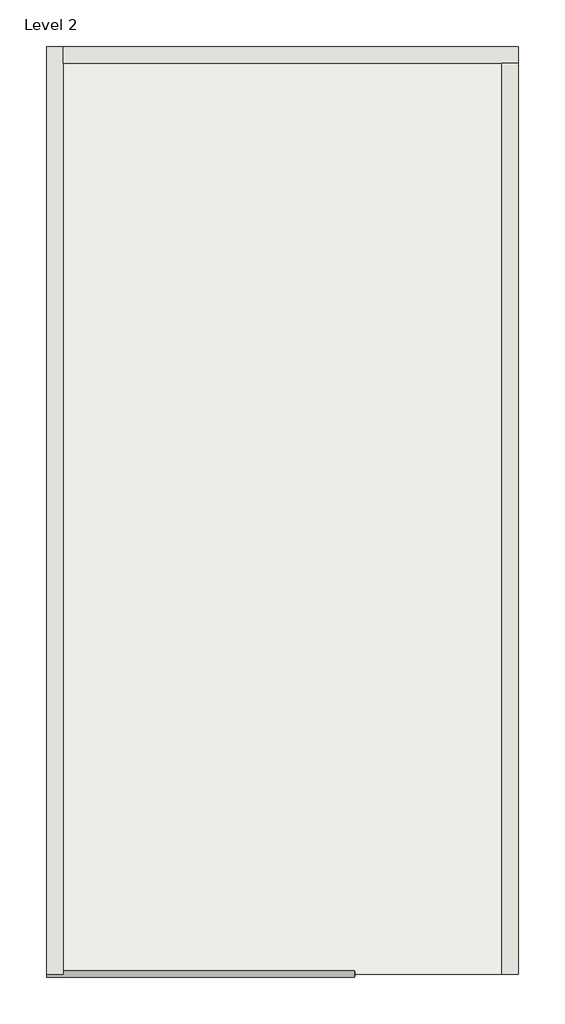
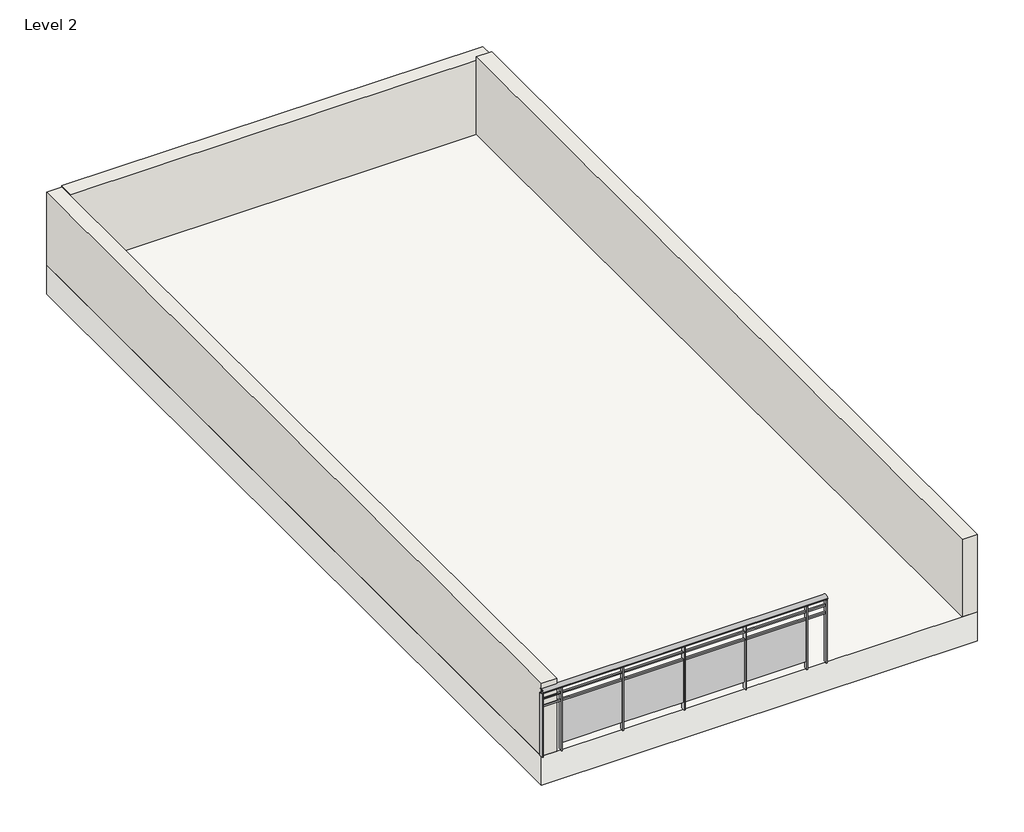
# One storey: 3 walls, 1 railing, 1 slab.
"""IFC4 building model written with IfcOpenShell, lengths in millimetres."""

from ifc_helpers import new_model, si_unit, point, frame, origin, place, context, project, spatial, polyline, ellipse_curve, trimmed, outline, extrude, faceted_brep, element, save
from ifc_brep_helpers import plane_surface, extruded_surface, advanced_brep

model = new_model("IFC4")

# Units and contexts
model_context = context("Model", 3, world=origin())
ifc_project = project(units=[si_unit("LENGTHUNIT", "METRE", prefix="MILLI")], contexts=[model_context])

# Site, building, storey
site = spatial("IfcSite", under=ifc_project)
building = spatial("IfcBuilding", under=site)
storey = spatial("IfcBuildingStorey", under=building, Name="Level 2", Elevation=6096.0)

# Railing
placement = place(None, origin())
element("IfcRailing", 1, ObjectType="Glass Panel - Bottom Fill", at=placement, inside=storey, context=model_context, shape_type="SolidModel", body=[
    advanced_brep(
    [(-9880.3407032, 3900.3863751, 6996.0), (-9880.3407032, 3820.3863751, 6996.0), (-6171.9407032, 3900.3863751, 6996.0), (-6171.9407032, 3820.3863751, 6996.0)],
    [
        (0, 1, ellipse_curve(frame((-9880.3407032, 3860.3863751, 6996.0), z_axis=(-1.0, 0.0, 0.0), x_axis=(0.0, -1.0, 0.0)), 40.0, 30.0)),
        (1, 0, ellipse_curve(frame((-9880.3407032, 3860.3863751, 6996.0), z_axis=(-1.0, 0.0, 0.0), x_axis=(0.0, -1.0, 0.0)), 40.0, 30.0)),
        (2, 3, ellipse_curve(frame((-6171.9407032, 3860.3863751, 6996.0), z_axis=(1.0, 0.0, 0.0), x_axis=(0.0, -1.0, 0.0)), 40.0, 30.0)),
        (3, 2, ellipse_curve(frame((-6171.9407032, 3860.3863751, 6996.0), z_axis=(1.0, 0.0, 0.0), x_axis=(0.0, -1.0, 0.0)), 40.0, 30.0)),
        (0, 2),
        (3, 1),
    ],
    [
        plane_surface(frame((-9880.3407032, 3860.3863751, 6996.0), z_axis=(-1.0, 0.0, 0.0), x_axis=(0.0, 1.0, 0.0))),
        plane_surface(frame((-6171.9407032, 3860.3863751, 6996.0), z_axis=(1.0, 0.0, 0.0), x_axis=(0.0, 1.0, 0.0))),
        extruded_surface(trimmed(ellipse_curve(frame((-6171.9407032, 3860.3863751, 6996.0), z_axis=(-1.0, 0.0, 0.0), x_axis=(0.0, -1.0, 0.0)), 40.0, 30.0), [point((-6171.9407032, 3900.3863751, 6996.0))], [point((-6171.9407032, 3820.3863751, 6996.0))], True, "CARTESIAN"), (-3708.3999999999996, 0.0, 0.0), 3708.3999999999996),
        extruded_surface(trimmed(ellipse_curve(frame((-6171.9407032, 3860.3863751, 6996.0), z_axis=(-1.0, 0.0, 0.0), x_axis=(0.0, -1.0, 0.0)), 40.0, 30.0), [point((-6171.9407032, 3820.3863751, 6996.0))], [point((-6171.9407032, 3900.3863751, 6996.0))], True, "CARTESIAN"), (-3708.3999999999996, 0.0, 0.0), 3708.3999999999996),
    ],
    [
        (0, [[1, 2]]),
        (1, [[3, 4]]),
        (2, [[-1, 5, -4, 6]]),
        (3, [[-2, -6, -3, -5]]),
    ],
),
    extrude(outline(polyline([(-9880.3407032, 3850.9956099), (-9880.3407032, 3870.9956099), (-6171.9407032, 3870.9956099), (-6171.9407032, 3850.9956099), (-9880.3407032, 3850.9956099)])), frame((0.0, 0.0, 6876.0), z_axis=(0.0, 0.0, 1.0), x_axis=(1.0, 0.0, 0.0)), (0.0, 0.0, 1.0), 20.0),
    extrude(outline(polyline([(-9880.3407032, 3850.9956099), (-9880.3407032, 3870.9956099), (-6171.9407032, 3870.9956099), (-6171.9407032, 3850.9956099), (-9880.3407032, 3850.9956099)])), frame((0.0, 0.0, 6776.0), z_axis=(0.0, 0.0, 1.0), x_axis=(1.0, 0.0, 0.0)), (0.0, 0.0, 1.0), 20.0),
    extrude(outline(polyline([(-6432.1407032, 3885.9956099), (-6420.1407032, 3885.9956099), (-6420.1407032, 3835.9956099), (-6432.1407032, 3835.9956099), (-6432.1407032, 3885.9956099)])), frame((0.0, 0.0, 6096.0), z_axis=(0.0, 0.0, 1.0), x_axis=(1.0, 0.0, 0.0)), (0.0, 0.0, 1.0), 869.8465326),
    extrude(outline(polyline([(-7226.1407032, 3859.2707998), (-6426.1407032, 3859.2707998), (-6426.1407032, 3854.2707998), (-7226.1407032, 3854.2707998), (-7226.1407032, 3859.2707998)])), frame((0.0, 0.0, 6196.0), z_axis=(0.0, 0.0, 1.0), x_axis=(1.0, 0.0, 0.0)), (0.0, 0.0, 1.0), 580.0),
    extrude(outline(polyline([(-7232.1407032, 3885.9956099), (-7220.1407032, 3885.9956099), (-7220.1407032, 3835.9956099), (-7232.1407032, 3835.9956099), (-7232.1407032, 3885.9956099)])), frame((0.0, 0.0, 6096.0), z_axis=(0.0, 0.0, 1.0), x_axis=(1.0, 0.0, 0.0)), (0.0, 0.0, 1.0), 869.8465326),
    extrude(outline(polyline([(-8026.1407032, 3859.2707998), (-7226.1407032, 3859.2707998), (-7226.1407032, 3854.2707998), (-8026.1407032, 3854.2707998), (-8026.1407032, 3859.2707998)])), frame((0.0, 0.0, 6196.0), z_axis=(0.0, 0.0, 1.0), x_axis=(1.0, 0.0, 0.0)), (0.0, 0.0, 1.0), 580.0),
    extrude(outline(polyline([(-8032.1407032, 3885.9956099), (-8020.1407032, 3885.9956099), (-8020.1407032, 3835.9956099), (-8032.1407032, 3835.9956099), (-8032.1407032, 3885.9956099)])), frame((0.0, 0.0, 6096.0), z_axis=(0.0, 0.0, 1.0), x_axis=(1.0, 0.0, 0.0)), (0.0, 0.0, 1.0), 869.8465326),
    extrude(outline(polyline([(-8826.1407032, 3859.2707998), (-8026.1407032, 3859.2707998), (-8026.1407032, 3854.2707998), (-8826.1407032, 3854.2707998), (-8826.1407032, 3859.2707998)])), frame((0.0, 0.0, 6196.0), z_axis=(0.0, 0.0, 1.0), x_axis=(1.0, 0.0, 0.0)), (0.0, 0.0, 1.0), 580.0),
    extrude(outline(polyline([(-8832.1407032, 3885.9956099), (-8820.1407032, 3885.9956099), (-8820.1407032, 3835.9956099), (-8832.1407032, 3835.9956099), (-8832.1407032, 3885.9956099)])), frame((0.0, 0.0, 6096.0), z_axis=(0.0, 0.0, 1.0), x_axis=(1.0, 0.0, 0.0)), (0.0, 0.0, 1.0), 869.8465326),
    extrude(outline(polyline([(-9626.1407032, 3859.2707998), (-8826.1407032, 3859.2707998), (-8826.1407032, 3854.2707998), (-9626.1407032, 3854.2707998), (-9626.1407032, 3859.2707998)])), frame((0.0, 0.0, 6196.0), z_axis=(0.0, 0.0, 1.0), x_axis=(1.0, 0.0, 0.0)), (0.0, 0.0, 1.0), 580.0),
    extrude(outline(polyline([(-9632.1407032, 3885.9956099), (-9620.1407032, 3885.9956099), (-9620.1407032, 3835.9956099), (-9632.1407032, 3835.9956099), (-9632.1407032, 3885.9956099)])), frame((0.0, 0.0, 6096.0), z_axis=(0.0, 0.0, 1.0), x_axis=(1.0, 0.0, 0.0)), (0.0, 0.0, 1.0), 869.8465326),
    extrude(outline(polyline([(-6179.9407032, 3885.9956099), (-6167.9407032, 3885.9956099), (-6167.9407032, 3835.9956099), (-6179.9407032, 3835.9956099), (-6179.9407032, 3885.9956099)])), frame((0.0, 0.0, 6096.0), z_axis=(0.0, 0.0, 1.0), x_axis=(1.0, 0.0, 0.0)), (0.0, 0.0, 1.0), 869.8465326),
    extrude(outline(polyline([(-9884.3407032, 3885.9956099), (-9872.3407032, 3885.9956099), (-9872.3407032, 3835.9956099), (-9884.3407032, 3835.9956099), (-9884.3407032, 3885.9956099)])), frame((0.0, 0.0, 6096.0), z_axis=(0.0, 0.0, 1.0), x_axis=(1.0, 0.0, 0.0)), (0.0, 0.0, 1.0), 869.8465326),
])

# Slab
element("IfcSlab", 2, ObjectType="Generic Floor - 400mm", at=placement, inside=storey, context=model_context, shape_type="SweptSolid", body=[
    extrude(outline(polyline([(-4193.9407032, 15033.7956099), (-4193.9407032, 3860.9956099), (-9880.3407032, 3860.9956099), (-9880.3407032, 15033.7956099), (-4193.9407032, 15033.7956099)])), frame((0.0, 0.0, 5696.0), z_axis=(0.0, 0.0, 1.0), x_axis=(1.0, 0.0, 0.0)), (0.0, 0.0, 1.0), 400.0),
])

# Walls
element("IfcWall", 3, ObjectType="Generic - 9\"", at=placement, inside=storey, context=model_context, shape_type="Brep", body=[
    faceted_brep([(-9680.3407032, 3860.9956099, 6096.0), (-9680.3407032, 14833.7956099, 6096.0), (-9680.3407032, 15033.7956099, 6096.0), (-9680.3407032, 15033.7956099, 7100.9541651), (-9680.3407032, 3860.9956099, 7100.9541651), (-9880.3407032, 3860.9956099, 6096.0), (-9880.3407032, 3860.9956099, 7100.9541651), (-9880.3407032, 15033.7956099, 7100.9541651), (-9880.3407032, 15033.7956099, 6096.0)], [[[0, 1, 2, 3, 4]], [[5, 6, 7, 8]], [[2, 1, 0, 5, 8]], [[4, 3, 7, 6]], [[0, 4, 6, 5]], [[3, 2, 8, 7]]]),
])
element("IfcWall", 4, ObjectType="Generic - 9\"", at=placement, inside=storey, context=model_context, shape_type="Brep", body=[
    faceted_brep([(-9680.3407032, 14833.7956099, 6096.0), (-4393.9407032, 14833.7956099, 6096.0), (-4193.9407032, 14833.7956099, 6096.0), (-4193.9407032, 14833.7956099, 7117.4757434), (-9680.3407032, 14833.7956099, 7117.4757434), (-9680.3407032, 15033.7956099, 6096.0), (-9680.3407032, 15033.7956099, 7100.9541651), (-9680.3407032, 15033.7956099, 7117.4757434), (-4193.9407032, 15033.7956099, 7117.4757434), (-4193.9407032, 15033.7956099, 6096.0)], [[[0, 1, 2, 3, 4]], [[5, 6, 7, 8, 9]], [[2, 1, 0, 5, 9]], [[4, 3, 8, 7]], [[0, 4, 7, 6, 5]], [[3, 2, 9, 8]]]),
])
element("IfcWall", 5, ObjectType="Generic - 9\"", at=placement, inside=storey, context=model_context, shape_type="Brep", body=[
    faceted_brep([(-4393.9407032, 14833.7956099, 6096.0), (-4393.9407032, 3860.9956099, 6096.0), (-4393.9407032, 3860.9956099, 7166.0945319), (-4393.9407032, 14833.7956099, 7166.0945319), (-4193.9407032, 14833.7956099, 6096.0), (-4193.9407032, 14833.7956099, 7117.4757434), (-4193.9407032, 14833.7956099, 7166.0945319), (-4193.9407032, 3860.9956099, 7166.0945319), (-4193.9407032, 3860.9956099, 6096.0)], [[[0, 1, 2, 3]], [[4, 5, 6, 7, 8]], [[1, 0, 4, 8]], [[2, 1, 8, 7]], [[3, 2, 7, 6]], [[0, 3, 6, 5, 4]]]),
])

save(model, "model.ifc")

# Revit data of these elements
# Type "Glass Panel - Bottom Fill"
#   built-in parameter 1008612 = 0.019685 (stored number, unit not read)
#   built-in parameter 1008611 = 0.019685 (stored number, unit not read)
#   built-in parameter 1008609 = 0.902231 (stored number, unit not read)
#   built-in parameter 1008604 = 0.19685 (stored number, unit not read)
#   built-in parameter 1008603 = 0.164042 (stored number, unit not read)
#   Railing Height = 900 mm
#   built-in parameter 1008630 = 2
#   built-in parameter 1008610 = 2
# Type "Generic Floor - 400mm"
#   Function = 0
#   Layers, outside or top first: 400 mm no material (function 1)
# Type "Generic - 9\""
#   Layers, outside or top first: 200 mm no material (function 1)
# Element 1 (IfcRailing, "Glass Panel - Bottom Fill")
#   Phase Created = New Construction
#   Materials on its faces: "Metal - Stainless Steel,Polished", "Glass"
# Element 2 (IfcSlab, "Generic Floor - 400mm")
#   Height Offset From Level = 0 mm
#   Phase Created = New Construction
#   Materials on its faces: "Default Roof"
# Element 3 (IfcWall, "Generic - 9\"")
#   Top Offset = 0 mm
#   Base Offset = 0 mm
#   Unconnected Height = 1004.954 mm
#   wall height = 1004.954 mm
#   Phase Created = New Construction
#   Base Constraint = Level 2
#   Materials on its faces: "Default Wall"
# Element 4 (IfcWall, "Generic - 9\"")
#   Top Offset = 0 mm
#   Base Offset = 0 mm
#   Unconnected Height = 1021.476 mm
#   wall height = 1021.476 mm
#   Phase Created = New Construction
#   Base Constraint = Level 2
#   Materials on its faces: "Default Wall"
# Element 5 (IfcWall, "Generic - 9\"")
#   Top Offset = 0 mm
#   Base Offset = 0 mm
#   Unconnected Height = 1070.095 mm
#   wall height = 1070.095 mm
#   Phase Created = New Construction
#   Base Constraint = Level 2
#   Materials on its faces: "Default Wall"
# Materials
#   "Metal - Stainless Steel,Polished": class "Metal", colour RGB 189 187 185, transparency 0, Cost = 0
#   "Glass": class "Glass", colour RGB 218 227 224, transparency 0.85, Description = "Soda Lime Glass", Cost = 0
#   "Default Roof": colour RGB 80 80 80, transparency 0
#   "Default Wall": colour RGB 80 80 80, transparency 0
